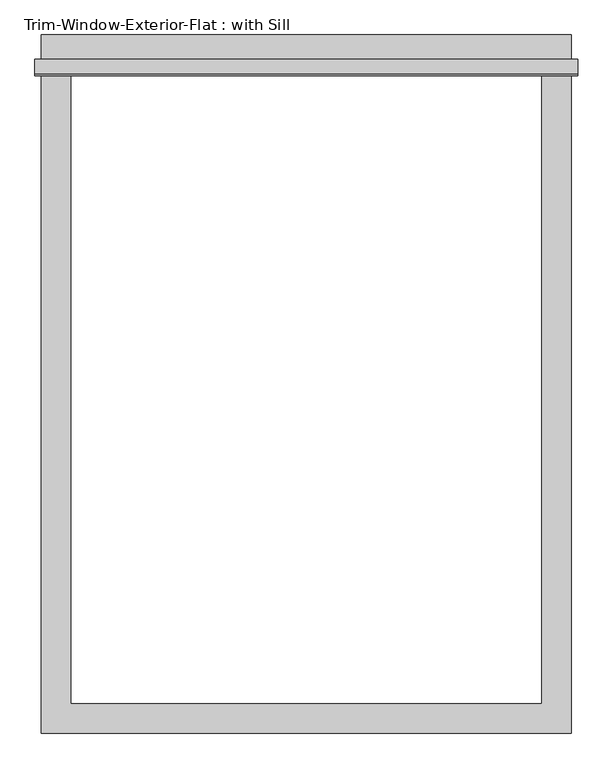
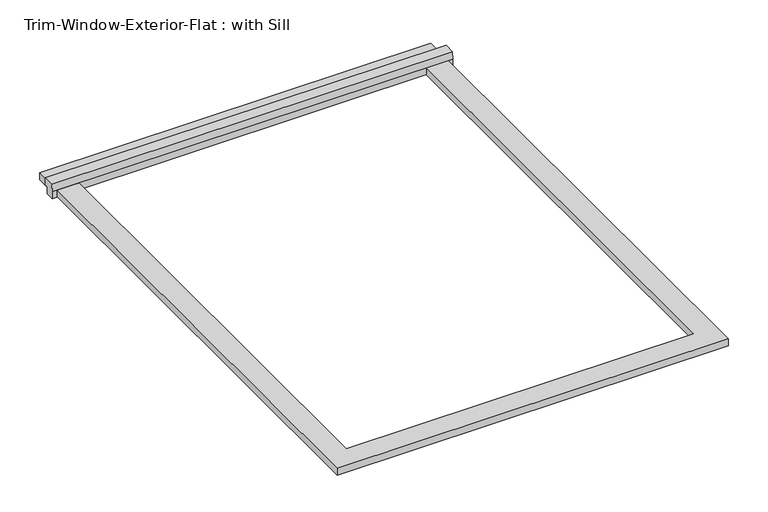
"""IFC4 building model written with IfcOpenShell, lengths in millimetres: proxy geometry, Trim-Window-Exterior-Flat : with Sill."""

from ifc_helpers import new_model, si_unit, frame, origin, origin_with_axes, place, context, project, spatial, polyline, outline, extrude, source, transform, mapped, element, save


def trim_window_exterior_flat_with_sill_80371c4b(model_context):
    return source(origin(), model_context, "Body", "SweptSolid", [
        extrude(outline(polyline([(514.35, 1241.3823709), (-514.35, 1241.3823709), (-514.35, 1298.5323709), (514.35, 1298.5323709), (514.35, 1241.3823709)])), origin_with_axes(), (0.0, 0.0, 1.0), 19.05),
        extrude(outline(polyline([(1250.95, 38.1), (1250.95, 19.05), (1241.3823709, 19.05), (1241.3823709, 0.0), (1219.2, 0.0), (1219.2, 19.05), (1221.6580645, 38.1), (1250.95, 38.1)])), frame((-527.05, 0.0, 0.0), z_axis=(1.0, 0.0, 0.0), x_axis=(0.0, 1.0, 0.0)), (0.0, 0.0, 1.0), 1054.1),
        extrude(outline(polyline([(-514.35, -57.15), (-514.35, 1219.2), (-457.2, 1219.2), (-457.2, 0.0), (457.2, 0.0), (457.2, 1219.2), (514.35, 1219.2), (514.35, -57.15), (-514.35, -57.15)])), origin_with_axes(), (0.0, 0.0, 1.0), 19.05),
    ])


if __name__ == "__main__":
    model = new_model("IFC4")
    model_context = context("Model", 3, world=origin())
    ifc_project = project(units=[si_unit("LENGTHUNIT", "METRE", prefix="MILLI")], contexts=[model_context])
    site = spatial("IfcSite", under=ifc_project)
    building = spatial("IfcBuilding", under=site)
    placement = place(None, origin())
    trim_window_exterior_flat_with_sill_shape = trim_window_exterior_flat_with_sill_80371c4b(model_context)
    element("IfcBuildingElementProxy", 1, Name="Trim-Window-Exterior-Flat : with Sill", ObjectType="Trim-Window-Exterior-Flat : with Sill", at=placement, inside=building, context=model_context, shape_type="MappedRepresentation", body=[
        mapped(trim_window_exterior_flat_with_sill_shape, transform((0.0, 0.0, 0.0), x_axis=(1.0, 0.0, 0.0), y_axis=(0.0, 1.0, 0.0), z_axis=(0.0, 0.0, 1.0))),
    ])
    save(model, "model.ifc")

# Revit data of these elements
# Type "Trim-Window-Exterior-Flat : with Sill"
#   Trim Width = 0' - 2 1/4"
#   Trim Thickness_Picture Frame = 0' - 1 1/4"
#   Trim Thickness_with Sill = 0' - 0 3/4"
#   Sill Thickness = 0' - 1 1/4"
#   Opening Width [instance default] = 2' - 0"
#   Opening Height [instance default] = 3' - 0"
#   Default Elevation = 4' - 0"
#   Sill = yes
#   Picture Frame = no
#   Trim Material [instance default] = none
# Element 1 (IfcBuildingElementProxy, "Trim-Window-Exterior-Flat : with Sill")
#   Opening Width = 3' - 0"
#   Opening Height = 4' - 0"
#   Trim Material = Clad - White
#   Materials on its faces: "Clad - White"
# Materials
#   "Clad - White": class "Wood", colour RGB 242 242 238, transparency 0, Cost = 0
